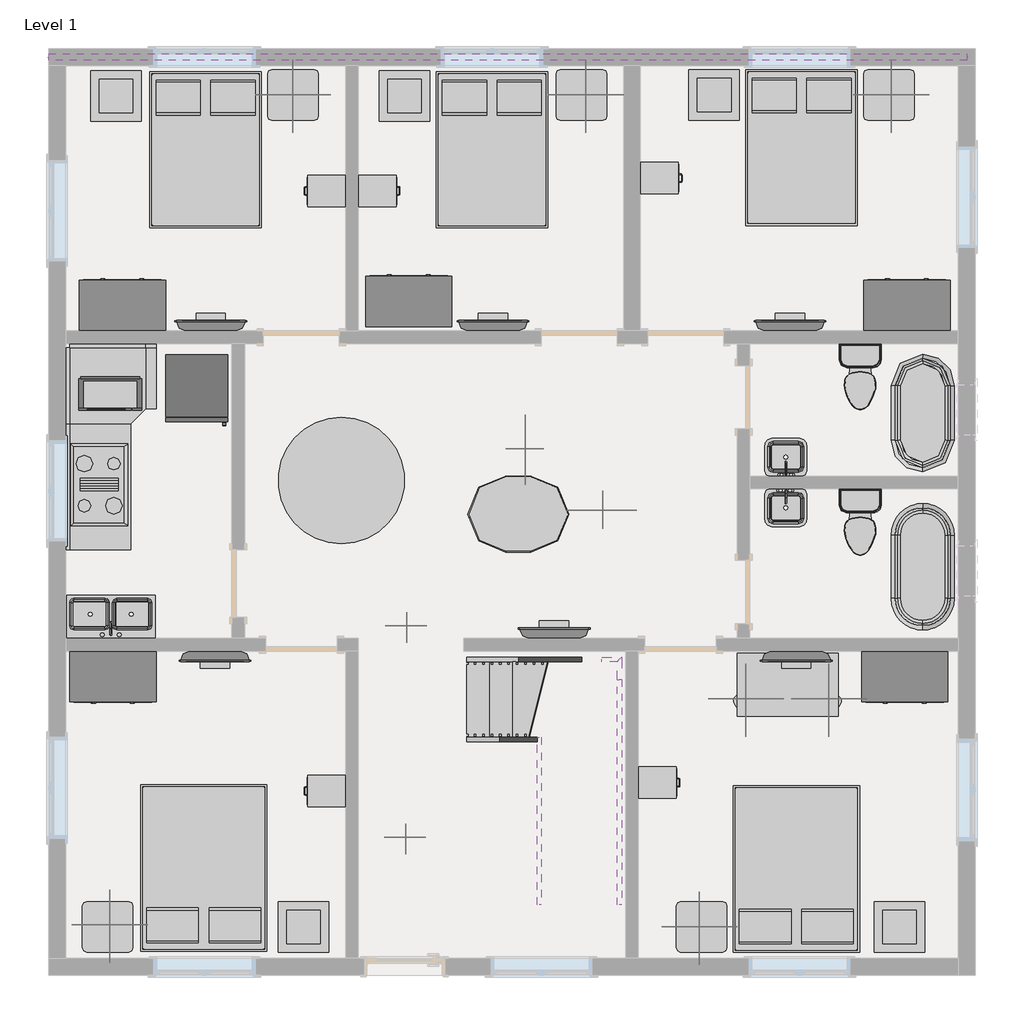
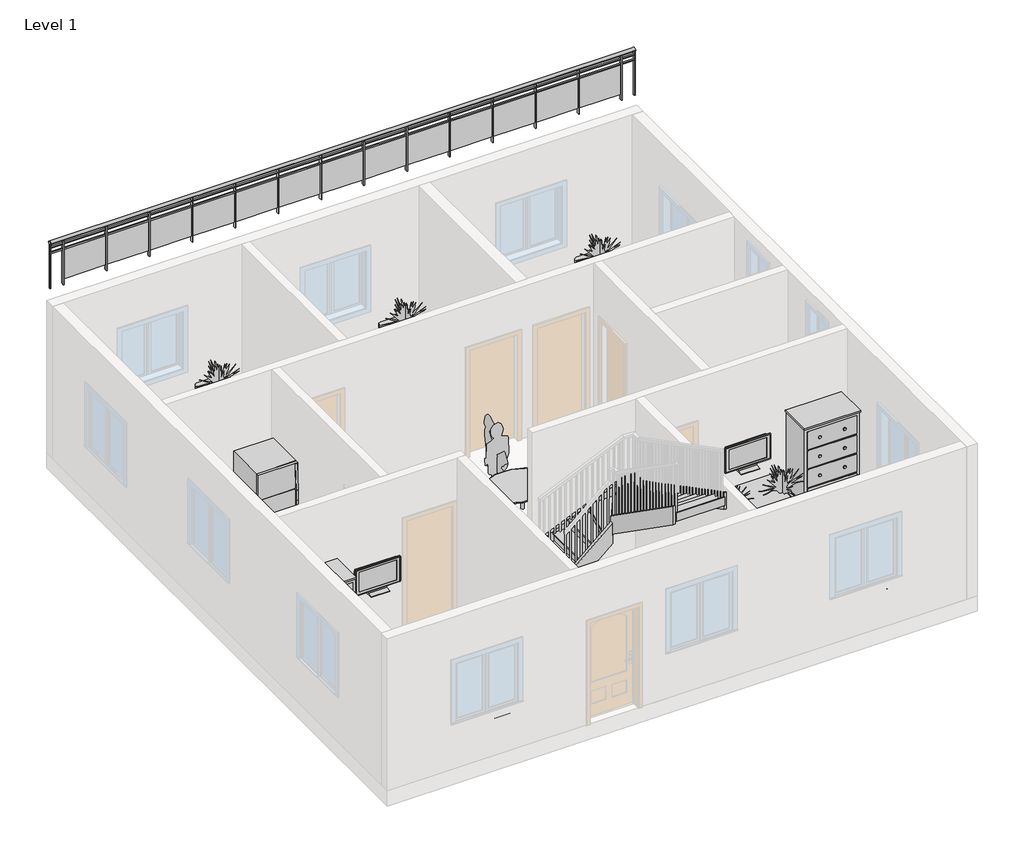
# One storey, part 3 of 3: 35 furniture elements, 9 flow terminals, 7 geographic elements, 7 proxies, 6 members, 1 railing, 1 stair flight.
"""IFC4 building model written with IfcOpenShell, lengths in millimetres."""

from ifc_helpers import new_model, si_unit, point, frame, origin, place, context, project, spatial, polyline, ellipse_curve, trimmed, outline, extrude, transform, mapped, element, save
from ifc_brep_helpers import plane_surface, extruded_surface, advanced_brep
from components import proxy_bb1e6e30, proxy_8a8d5ab2, rpc_female_69e001fa, rpc_male_28878092, proxy_a13a33b2, flow_terminal_2b63360b, flow_terminal_a53be723, flow_terminal_62a433f7, toilet_domestic_3d_toilet_domestic_3d_f7549cf7, toilet_domestic_3d_toilet_domestic_3d_183bbd19, flow_terminal_b374fae2, flow_terminal_a2f06f5b, furniture_c8abb964, furniture_1d2926bd, furniture_bb55ed6b, furniture_f72bdee3, furniture_56245f3a, furniture_b5c51a22, furniture_be1c6672, furniture_bbcc68ce, furniture_31d08a24, furniture_3f969c1c, furniture_6e13c3ce, rpc_plant_tropical_agave_1_5_93a2a214, stair_flight_d6903057

model = new_model("IFC4")

# Units and contexts
model_context = context("Model", 3, world=origin())
ifc_project = project(units=[si_unit("LENGTHUNIT", "METRE", prefix="MILLI")], contexts=[model_context])

# Site, building, storey
site = spatial("IfcSite", under=ifc_project)
building = spatial("IfcBuilding", under=site)
storey = spatial("IfcBuildingStorey", under=building, Name="Level 1", Elevation=0.0)

# Proxies
placement = place(None, origin())
proxy_shape = proxy_bb1e6e30(model_context)
element("IfcBuildingElementProxy", 1, Name="Cook Top-4 Unit : 36\" x 20\"", ObjectType="Cook Top-4 Unit : 36\" x 20\"", at=placement, inside=storey, context=model_context, shape_type="MappedRepresentation", body=[
    mapped(proxy_shape, transform((-16950.3067057, 8152.5187882, 0.0), x_axis=(0.0, 1.0000000000000002, 0.0), y_axis=(-1.0000000000000002, 0.0, 0.0), z_axis=(0.0, 0.0, 1.0))),
])
proxy_2_shape = proxy_8a8d5ab2(model_context)
element("IfcBuildingElementProxy", 2, Name="Microwave : 30\" x 16\" x 18\"", ObjectType="Microwave : 30\" x 16\" x 18\"", at=placement, inside=storey, context=model_context, shape_type="MappedRepresentation", body=[
    mapped(proxy_2_shape, transform((-17317.249583, 9604.149294, 0.0), x_axis=(1.0000000000000004, 0.0, 0.0), y_axis=(0.0, 1.0000000000000004, 0.0), z_axis=(0.0, 0.0, 1.0))),
])
rpc_female_shape = rpc_female_69e001fa(model_context)
element("IfcBuildingElementProxy", 3, Name="RPC Female", ObjectType="RPC Female", at=placement, inside=storey, context=model_context, shape_type="MappedRepresentation", body=[
    mapped(rpc_female_shape, transform((-11819.5067057, 8425.5687882, 0.0), x_axis=(1.0, 0.0, 0.0), y_axis=(0.0, 1.0, 0.0), z_axis=(0.0, 0.0, 1.0))),
])
element("IfcBuildingElementProxy", 4, Name="RPC Female", ObjectType="RPC Female", at=placement, inside=storey, context=model_context, shape_type="MappedRepresentation", body=[
    mapped(rpc_female_shape, transform((-11038.4567057, 7850.8434832, 0.0), x_axis=(0.0, -1.0000000000000004, 0.0), y_axis=(1.0000000000000004, 0.0, 0.0), z_axis=(0.0, 0.0, 1.0))),
])
rpc_male_shape = rpc_male_28878092(model_context)
element("IfcBuildingElementProxy", 5, Name="RPC Male", ObjectType="RPC Male", at=placement, inside=storey, context=model_context, shape_type="MappedRepresentation", body=[
    mapped(rpc_male_shape, transform((-13267.3067057, 3901.1937882, 0.0), x_axis=(1.0000000000000009, 0.0, 0.0), y_axis=(0.0, 1.0000000000000009, 0.0), z_axis=(0.0, 0.0, 1.0))),
])
element("IfcBuildingElementProxy", 6, Name="RPC Male", ObjectType="RPC Male", at=placement, inside=storey, context=model_context, shape_type="MappedRepresentation", body=[
    mapped(rpc_male_shape, transform((-13253.1160896, 6450.7187882, 0.0), x_axis=(1.0000000000000009, 0.0, 0.0), y_axis=(0.0, 1.0000000000000009, 0.0), z_axis=(0.0, 0.0, 1.0))),
])
proxy_3_shape = proxy_a13a33b2(model_context)
element("IfcBuildingElementProxy", 7, Name="Refrigerator : 30\" x 32\" RH", ObjectType="Refrigerator : 30\" x 32\" RH", at=placement, inside=storey, context=model_context, shape_type="MappedRepresentation", body=[
    mapped(proxy_3_shape, transform((-15774.3577342, 9328.8562882, 0.0), x_axis=(1.0000000000000007, 0.0, 0.0), y_axis=(0.0, 1.0000000000000007, 0.0), z_axis=(0.0, 0.0, 1.0))),
])

# Flow terminals
flow_terminal_shape = flow_terminal_2b63360b(model_context)
element("IfcFlowTerminal", 8, ObjectType="Floor Drain - Rectangular : 5\"x5\" Strainer - 2\" Drain", at=placement, inside=storey, context=model_context, shape_type="MappedRepresentation", body=[
    mapped(flow_terminal_shape, transform((-7692.0067057, 6552.3187882, 0.0), x_axis=(1.0, 0.0, 0.0), y_axis=(0.0, 1.0, 0.0), z_axis=(0.0, 0.0, 1.0))),
])
element("IfcFlowTerminal", 9, ObjectType="Floor Drain - Rectangular : 5\"x5\" Strainer - 2\" Drain", at=placement, inside=storey, context=model_context, shape_type="MappedRepresentation", body=[
    mapped(flow_terminal_shape, transform((-7628.5067057, 8457.3187882, 0.0), x_axis=(1.0, 0.0, 0.0), y_axis=(0.0, 1.0, 0.0), z_axis=(0.0, 0.0, 1.0))),
])
flow_terminal_2_shape = flow_terminal_a53be723(model_context)
element("IfcFlowTerminal", 10, ObjectType="Sink Kitchen-Double : 42\" x 21\"", at=placement, inside=storey, context=model_context, shape_type="MappedRepresentation", body=[
    mapped(flow_terminal_2_shape, transform((-16794.9174651, 6554.6641893, 0.0), x_axis=(-1.0000000000000002, 0.0, 0.0), y_axis=(0.0, -1.0000000000000002, 0.0), z_axis=(0.0, 0.0, 1.0))),
])
flow_terminal_3_shape = flow_terminal_62a433f7(model_context)
element("IfcFlowTerminal", 11, ObjectType="Sink Vanity-Square : 20\" x 18\"", at=placement, inside=storey, context=model_context, shape_type="MappedRepresentation", body=[
    mapped(flow_terminal_3_shape, transform((-8685.5959463, 7921.5733871, 0.0), x_axis=(1.0, 0.0, 0.0), y_axis=(0.0, 1.0, 0.0), z_axis=(0.0, 0.0, 1.0))),
])
element("IfcFlowTerminal", 12, ObjectType="Sink Vanity-Square : 20\" x 18\"", at=placement, inside=storey, context=model_context, shape_type="MappedRepresentation", body=[
    mapped(flow_terminal_3_shape, transform((-8654.2174651, 8434.2641893, 0.0), x_axis=(-1.0000000000000002, 0.0, 0.0), y_axis=(0.0, -1.0000000000000002, 0.0), z_axis=(0.0, 0.0, 1.0))),
])
toilet_domestic_3d_toilet_domestic_3d_shape = toilet_domestic_3d_toilet_domestic_3d_f7549cf7(model_context)
toilet_domestic_3d_toilet_domestic_3d_2_shape = toilet_domestic_3d_toilet_domestic_3d_183bbd19(model_context)
element("IfcFlowTerminal", 13, ObjectType="Toilet-Domestic-3D : Toilet-Domestic-3D", at=placement, inside=storey, context=model_context, shape_type="MappedRepresentation", body=[
    mapped(toilet_domestic_3d_toilet_domestic_3d_shape, transform((-7773.2107741, 7607.0227608, 0.0), x_axis=(1.0, 0.0, 0.0), y_axis=(0.0, 1.0, 0.0), z_axis=(0.0, 0.0, 1.0))),
    mapped(toilet_domestic_3d_toilet_domestic_3d_2_shape, transform((-7773.2107741, 7607.0227608, 0.0), x_axis=(1.0, 0.0, 0.0), y_axis=(0.0, 1.0, 0.0), z_axis=(0.0, 0.0, 1.0))),
])
element("IfcFlowTerminal", 14, ObjectType="Toilet-Domestic-3D : Toilet-Domestic-3D", at=placement, inside=storey, context=model_context, shape_type="MappedRepresentation", body=[
    mapped(toilet_domestic_3d_toilet_domestic_3d_shape, transform((-7773.2107741, 9359.6227608, 0.0), x_axis=(1.0, 0.0, 0.0), y_axis=(0.0, 1.0, 0.0), z_axis=(0.0, 0.0, 1.0))),
    mapped(toilet_domestic_3d_toilet_domestic_3d_2_shape, transform((-7773.2107741, 9359.6227608, 0.0), x_axis=(1.0, 0.0, 0.0), y_axis=(0.0, 1.0, 0.0), z_axis=(0.0, 0.0, 1.0))),
])
flow_terminal_4_shape = flow_terminal_b374fae2(model_context)
element("IfcFlowTerminal", 15, ObjectType="Tub-Free Standing-3D : 30\" x 60\"", at=placement, inside=storey, context=model_context, shape_type="MappedRepresentation", body=[
    mapped(flow_terminal_4_shape, transform((-7018.9067057, 7161.9187882, 0.0), x_axis=(1.0, 0.0, 0.0), y_axis=(0.0, 1.0, 0.0), z_axis=(0.0, 0.0, 1.0))),
])
flow_terminal_5_shape = flow_terminal_a2f06f5b(model_context)
element("IfcFlowTerminal", 16, ObjectType="Tub-Free Standing-3D : 30\" x 60\" 2", at=placement, inside=storey, context=model_context, shape_type="MappedRepresentation", body=[
    mapped(flow_terminal_5_shape, transform((-7018.9067057, 9016.1187882, 0.0), x_axis=(1.0, 0.0, 0.0), y_axis=(0.0, 1.0, 0.0), z_axis=(0.0, 0.0, 1.0))),
])

# Furniture
furniture_shape = furniture_c8abb964(model_context)
element("IfcFurniture", 17, ObjectType="Bed-Box : Double 53\" x 74\"", at=placement, inside=storey, context=model_context, shape_type="MappedRepresentation", body=[
    mapped(furniture_shape, transform((-16006.7591647, 12425.5482964, 0.0), x_axis=(1.0, 0.0, 0.0), y_axis=(0.0, 1.0, 0.0), z_axis=(0.0, 0.0, 1.0))),
])
element("IfcFurniture", 18, ObjectType="Bed-Box : Double 53\" x 74\"", at=placement, inside=storey, context=model_context, shape_type="MappedRepresentation", body=[
    mapped(furniture_shape, transform((-12552.3591647, 12425.5482964, 0.0), x_axis=(1.0, 0.0, 0.0), y_axis=(0.0, 1.0, 0.0), z_axis=(0.0, 0.0, 1.0))),
])
element("IfcFurniture", 19, ObjectType="Bed-Box : Double 53\" x 74\"", at=placement, inside=storey, context=model_context, shape_type="MappedRepresentation", body=[
    mapped(furniture_shape, transform((-8818.5591647, 12450.9482964, 0.0), x_axis=(1.0, 0.0, 0.0), y_axis=(0.0, 1.0, 0.0), z_axis=(0.0, 0.0, 1.0))),
])
furniture_2_shape = furniture_1d2926bd(model_context)
element("IfcFurniture", 20, ObjectType="Bed-Box : Queen 60\" x 79\"", at=placement, inside=storey, context=model_context, shape_type="MappedRepresentation", body=[
    mapped(furniture_2_shape, transform((-15350.1067057, 3295.28928, 0.0), x_axis=(-1.0000000000000002, 0.0, 0.0), y_axis=(0.0, -1.0000000000000002, 0.0), z_axis=(0.0, 0.0, 1.0))),
])
element("IfcFurniture", 21, ObjectType="Bed-Box : Queen 60\" x 79\"", at=placement, inside=storey, context=model_context, shape_type="MappedRepresentation", body=[
    mapped(furniture_2_shape, transform((-8203.7542467, 3282.58928, 0.0), x_axis=(-1.0, 0.0, 0.0), y_axis=(0.0, -1.0, 0.0), z_axis=(0.0, 0.0, 1.0))),
])
furniture_3_shape = furniture_bb55ed6b(model_context)
element("IfcFurniture", 22, ObjectType="Cabinet-File 2 Drawer : 15\" x 18\"", at=placement, inside=storey, context=model_context, shape_type="MappedRepresentation", body=[
    mapped(furniture_3_shape, transform((-14064.9724056, 11564.7774513, 0.0), x_axis=(0.0, -1.0000000000000002, 0.0), y_axis=(1.0000000000000002, 0.0, 0.0), z_axis=(0.0, 0.0, 1.0))),
])
element("IfcFurniture", 23, ObjectType="Cabinet-File 2 Drawer : 15\" x 18\"", at=placement, inside=storey, context=model_context, shape_type="MappedRepresentation", body=[
    mapped(furniture_3_shape, transform((-13739.6410058, 11823.7152352, 0.0), x_axis=(0.0, 1.0, 0.0), y_axis=(-1.0, 0.0, 0.0), z_axis=(0.0, 0.0, 1.0))),
])
element("IfcFurniture", 24, ObjectType="Cabinet-File 2 Drawer : 15\" x 18\"", at=placement, inside=storey, context=model_context, shape_type="MappedRepresentation", body=[
    mapped(furniture_3_shape, transform((-10336.0410058, 11976.1152352, 0.0), x_axis=(0.0, 1.0000000000000002, 0.0), y_axis=(-1.0000000000000002, 0.0, 0.0), z_axis=(0.0, 0.0, 1.0))),
])
element("IfcFurniture", 25, ObjectType="Cabinet-File 2 Drawer : 15\" x 18\"", at=placement, inside=storey, context=model_context, shape_type="MappedRepresentation", body=[
    mapped(furniture_3_shape, transform((-14064.9724056, 4328.9223411, 0.0), x_axis=(0.0, -1.0000000000000007, 0.0), y_axis=(1.0000000000000007, 0.0, 0.0), z_axis=(0.0, 0.0, 1.0))),
])
element("IfcFurniture", 26, ObjectType="Cabinet-File 2 Drawer : 15\" x 18\"", at=placement, inside=storey, context=model_context, shape_type="MappedRepresentation", body=[
    mapped(furniture_3_shape, transform((-10361.4410058, 4686.3152352, 0.0), x_axis=(0.0, 1.0, 0.0), y_axis=(-1.0, 0.0, 0.0), z_axis=(0.0, 0.0, 1.0))),
])
furniture_4_shape = furniture_f72bdee3(model_context)
element("IfcFurniture", 27, ObjectType="Dresser : 48\" x 72\" x 24\"", at=placement, inside=storey, context=model_context, shape_type="MappedRepresentation", body=[
    mapped(furniture_4_shape, transform((-16940.0999656, 9948.3558341, 0.0), x_axis=(-1.0000000000000004, 0.0, 0.0), y_axis=(0.0, -1.0000000000000004, 0.0), z_axis=(0.0, 0.0, 1.0))),
])
element("IfcFurniture", 28, ObjectType="Dresser : 48\" x 72\" x 24\"", at=placement, inside=storey, context=model_context, shape_type="MappedRepresentation", body=[
    mapped(furniture_4_shape, transform((-13485.6999656, 9999.1558341, 0.0), x_axis=(-1.0000000000000004, 0.0, 0.0), y_axis=(0.0, -1.0000000000000004, 0.0), z_axis=(0.0, 0.0, 1.0))),
])
element("IfcFurniture", 29, ObjectType="Dresser : 48\" x 72\" x 24\"", at=placement, inside=storey, context=model_context, shape_type="MappedRepresentation", body=[
    mapped(furniture_4_shape, transform((-7478.5999656, 9948.3558341, 0.0), x_axis=(-1.0000000000000004, 0.0, 0.0), y_axis=(0.0, -1.0000000000000004, 0.0), z_axis=(0.0, 0.0, 1.0))),
])
element("IfcFurniture", 30, ObjectType="Dresser : 48\" x 72\" x 24\"", at=placement, inside=storey, context=model_context, shape_type="MappedRepresentation", body=[
    mapped(furniture_4_shape, transform((-16516.0134459, 6204.2817423, 0.0), x_axis=(1.0, 0.0, 0.0), y_axis=(0.0, 1.0, 0.0), z_axis=(0.0, 0.0, 1.0))),
])
element("IfcFurniture", 31, ObjectType="Dresser : 48\" x 72\" x 24\"", at=placement, inside=storey, context=model_context, shape_type="MappedRepresentation", body=[
    mapped(furniture_4_shape, transform((-6965.6134459, 6204.2817423, 0.0), x_axis=(1.0, 0.0, 0.0), y_axis=(0.0, 1.0, 0.0), z_axis=(0.0, 0.0, 1.0))),
])
furniture_5_shape = furniture_56245f3a(model_context)
element("IfcFurniture", 32, ObjectType="TV - Flat Screen : 32\"", at=placement, inside=storey, context=model_context, shape_type="MappedRepresentation", body=[
    mapped(furniture_5_shape, transform((-15608.0512199, 10065.2574118, 990.6), x_axis=(-1.0000000000000002, 0.0, 0.0), y_axis=(0.0, -1.0000000000000002, 0.0), z_axis=(0.0, 0.0, 1.0))),
])
element("IfcFurniture", 33, ObjectType="TV - Flat Screen : 32\"", at=placement, inside=storey, context=model_context, shape_type="MappedRepresentation", body=[
    mapped(furniture_5_shape, transform((-12204.4512199, 10065.2574118, 990.6), x_axis=(-1.0000000000000009, 0.0, 0.0), y_axis=(0.0, -1.0000000000000009, 0.0), z_axis=(0.0, 0.0, 1.0))),
])
element("IfcFurniture", 34, ObjectType="TV - Flat Screen : 32\"", at=placement, inside=storey, context=model_context, shape_type="MappedRepresentation", body=[
    mapped(furniture_5_shape, transform((-8623.0512199, 10065.2574118, 990.6), x_axis=(-1.0, 0.0, 0.0), y_axis=(0.0, -1.0, 0.0), z_axis=(0.0, 0.0, 1.0))),
])
element("IfcFurniture", 35, ObjectType="TV - Flat Screen : 32\"", at=placement, inside=storey, context=model_context, shape_type="MappedRepresentation", body=[
    mapped(furniture_5_shape, transform((-15549.3621916, 6087.3801645, 990.6), x_axis=(1.0, 0.0, 0.0), y_axis=(0.0, 1.0, 0.0), z_axis=(0.0, 0.0, 1.0))),
])
element("IfcFurniture", 36, ObjectType="TV - Flat Screen : 32\"", at=placement, inside=storey, context=model_context, shape_type="MappedRepresentation", body=[
    mapped(furniture_5_shape, transform((-8538.9621916, 6087.3801645, 990.6), x_axis=(1.0, 0.0, 0.0), y_axis=(0.0, 1.0, 0.0), z_axis=(0.0, 0.0, 1.0))),
])
element("IfcFurniture", 37, ObjectType="TV - Flat Screen : 32\"", at=placement, inside=storey, context=model_context, shape_type="MappedRepresentation", body=[
    mapped(furniture_5_shape, transform((-11467.8512199, 6356.8574118, 1092.2), x_axis=(-1.0000000000000002, 0.0, 0.0), y_axis=(0.0, -1.0000000000000002, 0.0), z_axis=(0.0, 0.0, 1.0))),
])
furniture_6_shape = furniture_b5c51a22(model_context)
element("IfcFurniture", 38, ObjectType="Table-Coffee : 24\" x 24\" x 24\"", at=placement, inside=storey, context=model_context, shape_type="MappedRepresentation", body=[
    mapped(furniture_6_shape, transform((-16765.3724724, 12743.6077104, 0.0), x_axis=(1.0, 0.0, 0.0), y_axis=(0.0, 1.0, 0.0), z_axis=(0.0, 0.0, 1.0))),
])
element("IfcFurniture", 39, ObjectType="Table-Coffee : 24\" x 24\" x 24\"", at=placement, inside=storey, context=model_context, shape_type="MappedRepresentation", body=[
    mapped(furniture_6_shape, transform((-13285.5724724, 12743.6077104, 0.0), x_axis=(1.0, 0.0, 0.0), y_axis=(0.0, 1.0, 0.0), z_axis=(0.0, 0.0, 1.0))),
])
element("IfcFurniture", 40, ObjectType="Table-Coffee : 24\" x 24\" x 24\"", at=placement, inside=storey, context=model_context, shape_type="MappedRepresentation", body=[
    mapped(furniture_6_shape, transform((-9551.7724724, 12756.3077104, 0.0), x_axis=(1.0, 0.0, 0.0), y_axis=(0.0, 1.0, 0.0), z_axis=(0.0, 0.0, 1.0))),
])
element("IfcFurniture", 41, ObjectType="Table-Coffee : 24\" x 24\" x 24\"", at=placement, inside=storey, context=model_context, shape_type="MappedRepresentation", body=[
    mapped(furniture_6_shape, transform((-14504.7724724, 2723.3077104, 0.0), x_axis=(1.0, 0.0, 0.0), y_axis=(0.0, 1.0, 0.0), z_axis=(0.0, 0.0, 1.0))),
])
element("IfcFurniture", 42, ObjectType="Table-Coffee : 24\" x 24\" x 24\"", at=placement, inside=storey, context=model_context, shape_type="MappedRepresentation", body=[
    mapped(furniture_6_shape, transform((-7316.5724724, 2723.3077104, 0.0), x_axis=(1.0, 0.0, 0.0), y_axis=(0.0, 1.0, 0.0), z_axis=(0.0, 0.0, 1.0))),
])
furniture_7_shape = furniture_be1c6672(model_context)
element("IfcFurniture", 43, ObjectType="Table-Dining Oval : 36\" x 48\"", at=placement, inside=storey, context=model_context, shape_type="MappedRepresentation", body=[
    mapped(furniture_7_shape, transform((-11493.8870336, 8155.0171488, 0.0), x_axis=(1.0, 0.0, 0.0), y_axis=(0.0, 1.0, 0.0), z_axis=(0.0, 0.0, 1.0))),
])
furniture_8_shape = furniture_bbcc68ce(model_context)
element("IfcFurniture", 44, ObjectType="Table-Dining Round w Chairs : 60\" Diameter", at=placement, inside=storey, context=model_context, shape_type="MappedRepresentation", body=[
    mapped(furniture_8_shape, transform((-14132.9886729, 8388.1974767, 0.0), x_axis=(1.0, 0.0, 0.0), y_axis=(0.0, 1.0, 0.0), z_axis=(0.0, 0.0, 1.0))),
])
furniture_9_shape = furniture_31d08a24(model_context)
element("IfcFurniture", 45, ObjectType="Table-End : 24\" x 24\"", at=placement, inside=storey, context=model_context, shape_type="MappedRepresentation", body=[
    mapped(furniture_9_shape, transform((-14922.040336, 12699.1187882, 0.0), x_axis=(1.0, 0.0, 0.0), y_axis=(0.0, 1.0, 0.0), z_axis=(0.0, 0.0, 1.0))),
])
element("IfcFurniture", 46, ObjectType="Table-End : 24\" x 24\"", at=placement, inside=storey, context=model_context, shape_type="MappedRepresentation", body=[
    mapped(furniture_9_shape, transform((-11442.240336, 12699.1187882, 0.0), x_axis=(1.0, 0.0, 0.0), y_axis=(0.0, 1.0, 0.0), z_axis=(0.0, 0.0, 1.0))),
])
element("IfcFurniture", 47, ObjectType="Table-End : 24\" x 24\"", at=placement, inside=storey, context=model_context, shape_type="MappedRepresentation", body=[
    mapped(furniture_9_shape, transform((-7733.840336, 12699.1187882, 0.0), x_axis=(1.0, 0.0, 0.0), y_axis=(0.0, 1.0, 0.0), z_axis=(0.0, 0.0, 1.0))),
])
element("IfcFurniture", 48, ObjectType="Table-End : 24\" x 24\"", at=placement, inside=storey, context=model_context, shape_type="MappedRepresentation", body=[
    mapped(furniture_9_shape, transform((-17157.240336, 2666.1187882, 0.0), x_axis=(1.0, 0.0, 0.0), y_axis=(0.0, 1.0, 0.0), z_axis=(0.0, 0.0, 1.0))),
])
element("IfcFurniture", 49, ObjectType="Table-End : 24\" x 24\"", at=placement, inside=storey, context=model_context, shape_type="MappedRepresentation", body=[
    mapped(furniture_9_shape, transform((-9994.440336, 2666.1187882, 0.0), x_axis=(1.0, 0.0, 0.0), y_axis=(0.0, 1.0, 0.0), z_axis=(0.0, 0.0, 1.0))),
])
furniture_10_shape = furniture_3f969c1c(model_context)
element("IfcFurniture", 50, ObjectType="Table-Rectangular : 72\" x 30\"", at=placement, inside=storey, context=model_context, shape_type="MappedRepresentation", body=[
    mapped(furniture_10_shape, transform((-8644.5067057, 5739.5187882, 0.0), x_axis=(1.0, 0.0, 0.0), y_axis=(0.0, 1.0, 0.0), z_axis=(0.0, 0.0, 1.0))),
])
furniture_11_shape = furniture_6e13c3ce(model_context)
element("IfcFurniture", 51, ObjectType="Work Station Cubicle : 96\" x 96\"", at=placement, inside=storey, context=model_context, shape_type="MappedRepresentation", body=[
    mapped(furniture_11_shape, transform((-17224.9749535, 10349.3417958, 0.0), x_axis=(1.0, 0.0, 0.0), y_axis=(0.0, 1.0, 0.0), z_axis=(0.0, 0.0, 1.0))),
])

# Geographic elements
rpc_plant_tropical_agave_1_5_shape = rpc_plant_tropical_agave_1_5_93a2a214(model_context)
element("IfcGeographicElement", 52, ObjectType="RPC Plant - Tropical : Agave - 1.5'", at=placement, inside=storey, context=model_context, shape_type="MappedRepresentation", body=[
    mapped(rpc_plant_tropical_agave_1_5_shape, transform((-14613.5067057, 12851.5187882, 609.6), x_axis=(1.0, 0.0, 0.0), y_axis=(0.0, 1.0, 0.0), z_axis=(0.0, 0.0, 1.0))),
])
element("IfcGeographicElement", 53, ObjectType="RPC Plant - Tropical : Agave - 1.5'", at=placement, inside=storey, context=model_context, shape_type="MappedRepresentation", body=[
    mapped(rpc_plant_tropical_agave_1_5_shape, transform((-11082.9067057, 12851.5187882, 609.6), x_axis=(1.0, 0.0, 0.0), y_axis=(0.0, 1.0, 0.0), z_axis=(0.0, 0.0, 1.0))),
])
element("IfcGeographicElement", 54, ObjectType="RPC Plant - Tropical : Agave - 1.5'", at=placement, inside=storey, context=model_context, shape_type="MappedRepresentation", body=[
    mapped(rpc_plant_tropical_agave_1_5_shape, transform((-7399.9067057, 12851.5187882, 609.6), x_axis=(1.0, 0.0, 0.0), y_axis=(0.0, 1.0, 0.0), z_axis=(0.0, 0.0, 1.0))),
])
element("IfcGeographicElement", 55, ObjectType="RPC Plant - Tropical : Agave - 1.5'", at=placement, inside=storey, context=model_context, shape_type="MappedRepresentation", body=[
    mapped(rpc_plant_tropical_agave_1_5_shape, transform((-16823.3067057, 2843.9187882, 609.6), x_axis=(1.0, 0.0, 0.0), y_axis=(0.0, 1.0, 0.0), z_axis=(0.0, 0.0, 1.0))),
])
element("IfcGeographicElement", 56, ObjectType="RPC Plant - Tropical : Agave - 1.5'", at=placement, inside=storey, context=model_context, shape_type="MappedRepresentation", body=[
    mapped(rpc_plant_tropical_agave_1_5_shape, transform((-9711.3067057, 2818.5187882, 609.6), x_axis=(1.0, 0.0, 0.0), y_axis=(0.0, 1.0, 0.0), z_axis=(0.0, 0.0, 1.0))),
])
element("IfcGeographicElement", 57, ObjectType="RPC Plant - Tropical : Agave - 1.5'", at=placement, inside=storey, context=model_context, shape_type="MappedRepresentation", body=[
    mapped(rpc_plant_tropical_agave_1_5_shape, transform((-8149.2067057, 5568.0687882, 660.4), x_axis=(1.0, 0.0, 0.0), y_axis=(0.0, 1.0, 0.0), z_axis=(0.0, 0.0, 1.0))),
])
element("IfcGeographicElement", 58, ObjectType="RPC Plant - Tropical : Agave - 1.5'", at=placement, inside=storey, context=model_context, shape_type="MappedRepresentation", body=[
    mapped(rpc_plant_tropical_agave_1_5_shape, transform((-9152.5067057, 5568.0687882, 660.4), x_axis=(1.0, 0.0, 0.0), y_axis=(0.0, 1.0, 0.0), z_axis=(0.0, 0.0, 1.0))),
])

# Members
element("IfcMember", 59, ObjectType="Stringer - 2\" Width", at=placement, inside=storey, context=model_context, shape_type="SweptSolid", body=[
    extrude(outline(polyline([(922.8849999, -12520.2436952), (590.0562463, -12520.2436952), (1305.2683876, -10889.5815024), (1638.0971411, -10889.5815024), (922.8849999, -12520.2436952)])), frame((0.0, 6018.9187882, 0.0), z_axis=(0.0, 1.0, 0.0), x_axis=(0.0, 0.0, 1.0)), (0.0, 0.0, 1.0), 50.8),
])
element("IfcMember", 60, ObjectType="Stringer - 2\" Width", at=placement, inside=storey, context=model_context, shape_type="SweptSolid", body=[
    extrude(outline(polyline([(-10889.5815024, 6018.9187882), (-10889.5815024, 6069.7187882), (-10651.1067057, 6069.7187882), (-10701.9067057, 6018.9187882), (-10889.5815024, 6018.9187882)])), frame((0.0, 0.0, 1305.2683876), z_axis=(0.0, 0.0, 1.0), x_axis=(1.0, 0.0, 0.0)), (0.0, 0.0, 1.0), 332.8287535),
])
element("IfcMember", 61, ObjectType="Stringer - 2\" Width", at=placement, inside=storey, context=model_context, shape_type="SweptSolid", body=[
    extrude(outline(polyline([(-10701.9067057, 6018.9187882), (-10651.1067057, 6069.7187882), (-10651.1067057, 5800.7654451), (-10701.9067057, 5800.7654451), (-10701.9067057, 6018.9187882)])), frame((0.0, 0.0, 1305.2683876), z_axis=(0.0, 0.0, 1.0), x_axis=(1.0, 0.0, 0.0)), (0.0, 0.0, 1.0), 332.8287535),
])
element("IfcMember", 62, ObjectType="Stringer - 2\" Width", at=placement, inside=storey, context=model_context, shape_type="SweptSolid", body=[
    extrude(outline(polyline([(5800.7654451, 1638.0971411), (5800.7654451, 1305.2683876), (3082.9817987, 2720.7901969), (3082.9817987, 3053.6189504), (5800.7654451, 1638.0971411)])), frame((-10701.9067057, 0.0, 0.0), z_axis=(1.0, 0.0, 0.0), x_axis=(0.0, 1.0, 0.0)), (0.0, 0.0, 1.0), 50.8),
])
element("IfcMember", 63, ObjectType="Stringer - 2\" Width", at=placement, inside=storey, context=model_context, shape_type="SweptSolid", body=[
    extrude(outline(polyline([(842.634734, -12520.2436952), (435.4922729, -12520.2436952), (1191.0265733, -11667.1067057), (1598.1690344, -11667.1067057), (842.634734, -12520.2436952)])), frame((0.0, 5053.7187882, 0.0), z_axis=(0.0, 1.0, 0.0), x_axis=(0.0, 0.0, 1.0)), (0.0, 0.0, 1.0), 50.8),
])
element("IfcMember", 64, ObjectType="Stringer - 2\" Width", at=placement, inside=storey, context=model_context, shape_type="SweptSolid", body=[
    extrude(outline(polyline([(5104.5187882, 1709.9296678), (5104.5187882, 1337.7212805), (3082.9817987, 2754.5609981), (3082.9817987, 3126.7693854), (5104.5187882, 1709.9296678)])), frame((-11667.1067057, 0.0, 0.0), z_axis=(1.0, 0.0, 0.0), x_axis=(0.0, 1.0, 0.0)), (0.0, 0.0, 1.0), 50.8),
])

# Railing
element("IfcRailing", 65, ObjectType="Glass Panel - Bottom Fill", at=placement, inside=storey, context=model_context, shape_type="SolidModel", body=[
    advanced_brep(
    [(-17559.9067057, 13346.8187882, 4267.2), (-17559.9067057, 13270.6187882, 4267.2), (-6485.5067057, 13346.8187882, 4267.2), (-6485.5067057, 13270.6187882, 4267.2)],
    [
        (0, 1, ellipse_curve(frame((-17559.9067057, 13308.7187882, 4267.2), z_axis=(-1.0, 0.0, 0.0), x_axis=(0.0, -1.0, 0.0)), 38.1, 28.575)),
        (1, 0, ellipse_curve(frame((-17559.9067057, 13308.7187882, 4267.2), z_axis=(-1.0, 0.0, 0.0), x_axis=(0.0, -1.0, 0.0)), 38.1, 28.575)),
        (2, 3, ellipse_curve(frame((-6485.5067057, 13308.7187882, 4267.2), z_axis=(1.0, 0.0, 0.0), x_axis=(0.0, -1.0, 0.0)), 38.1, 28.575)),
        (3, 2, ellipse_curve(frame((-6485.5067057, 13308.7187882, 4267.2), z_axis=(1.0, 0.0, 0.0), x_axis=(0.0, -1.0, 0.0)), 38.1, 28.575)),
        (0, 2),
        (3, 1),
    ],
    [
        plane_surface(frame((-17559.9067057, 13308.7187882, 4267.2), z_axis=(-1.0, 0.0, 0.0), x_axis=(0.0, 1.0, 0.0))),
        plane_surface(frame((-6485.5067057, 13308.7187882, 4267.2), z_axis=(1.0, 0.0, 0.0), x_axis=(0.0, 1.0, 0.0))),
        extruded_surface(trimmed(ellipse_curve(frame((-6485.5067057, 13308.7187882, 4267.2), z_axis=(-1.0, 0.0, 0.0), x_axis=(0.0, -1.0, 0.0)), 38.1, 28.575), [point((-6485.5067057, 13346.8187882, 4267.2))], [point((-6485.5067057, 13270.6187882, 4267.2))], True, "CARTESIAN"), (-11074.4, 0.0, 0.0), 11074.4),
        extruded_surface(trimmed(ellipse_curve(frame((-6485.5067057, 13308.7187882, 4267.2), z_axis=(-1.0, 0.0, 0.0), x_axis=(0.0, -1.0, 0.0)), 38.1, 28.575), [point((-6485.5067057, 13270.6187882, 4267.2))], [point((-6485.5067057, 13346.8187882, 4267.2))], True, "CARTESIAN"), (-11074.4, 0.0, 0.0), 11074.4),
    ],
    [
        (0, [[1, 2]]),
        (1, [[3, 4]]),
        (2, [[-1, 5, -4, 6]]),
        (3, [[-2, -6, -3, -5]]),
    ],
),
    extrude(outline(polyline([(-17559.9067057, 13296.0187882), (-17559.9067057, 13321.4187882), (-6485.5067057, 13321.4187882), (-6485.5067057, 13296.0187882), (-17559.9067057, 13296.0187882)])), frame((0.0, 0.0, 4152.9), z_axis=(0.0, 0.0, 1.0), x_axis=(1.0, 0.0, 0.0)), (0.0, 0.0, 1.0), 25.4),
    extrude(outline(polyline([(-17559.9067057, 13296.0187882), (-17559.9067057, 13321.4187882), (-6485.5067057, 13321.4187882), (-6485.5067057, 13296.0187882), (-17559.9067057, 13296.0187882)])), frame((0.0, 0.0, 4051.3), z_axis=(0.0, 0.0, 1.0), x_axis=(1.0, 0.0, 0.0)), (0.0, 0.0, 1.0), 25.4),
    extrude(outline(polyline([(-6745.8567057, 13283.3187882), (-6745.8567057, 13334.1187882), (-6733.1567057, 13334.1187882), (-6733.1567057, 13283.3187882), (-6745.8567057, 13283.3187882)])), frame((0.0, 0.0, 3352.8), z_axis=(0.0, 0.0, 1.0), x_axis=(1.0, 0.0, 0.0)), (0.0, 0.0, 1.0), 885.6788223),
    extrude(outline(polyline([(-7552.3067057, 13315.2539452), (-6739.5067057, 13315.2539452), (-6739.5067057, 13308.9039452), (-7552.3067057, 13308.9039452), (-7552.3067057, 13315.2539452)])), frame((0.0, 0.0, 3454.4), z_axis=(0.0, 0.0, 1.0), x_axis=(1.0, 0.0, 0.0)), (0.0, 0.0, 1.0), 596.9),
    extrude(outline(polyline([(-7558.6567057, 13283.3187882), (-7558.6567057, 13334.1187882), (-7545.9567057, 13334.1187882), (-7545.9567057, 13283.3187882), (-7558.6567057, 13283.3187882)])), frame((0.0, 0.0, 3352.8), z_axis=(0.0, 0.0, 1.0), x_axis=(1.0, 0.0, 0.0)), (0.0, 0.0, 1.0), 885.6788223),
    extrude(outline(polyline([(-8365.1067057, 13315.2539452), (-7552.3067057, 13315.2539452), (-7552.3067057, 13308.9039452), (-8365.1067057, 13308.9039452), (-8365.1067057, 13315.2539452)])), frame((0.0, 0.0, 3454.4), z_axis=(0.0, 0.0, 1.0), x_axis=(1.0, 0.0, 0.0)), (0.0, 0.0, 1.0), 596.9),
    extrude(outline(polyline([(-8371.4567057, 13283.3187882), (-8371.4567057, 13334.1187882), (-8358.7567057, 13334.1187882), (-8358.7567057, 13283.3187882), (-8371.4567057, 13283.3187882)])), frame((0.0, 0.0, 3352.8), z_axis=(0.0, 0.0, 1.0), x_axis=(1.0, 0.0, 0.0)), (0.0, 0.0, 1.0), 885.6788223),
    extrude(outline(polyline([(-9177.9067057, 13315.2539452), (-8365.1067057, 13315.2539452), (-8365.1067057, 13308.9039452), (-9177.9067057, 13308.9039452), (-9177.9067057, 13315.2539452)])), frame((0.0, 0.0, 3454.4), z_axis=(0.0, 0.0, 1.0), x_axis=(1.0, 0.0, 0.0)), (0.0, 0.0, 1.0), 596.9),
    extrude(outline(polyline([(-9184.2567057, 13283.3187882), (-9184.2567057, 13334.1187882), (-9171.5567057, 13334.1187882), (-9171.5567057, 13283.3187882), (-9184.2567057, 13283.3187882)])), frame((0.0, 0.0, 3352.8), z_axis=(0.0, 0.0, 1.0), x_axis=(1.0, 0.0, 0.0)), (0.0, 0.0, 1.0), 885.6788223),
    extrude(outline(polyline([(-9990.7067057, 13315.2539452), (-9177.9067057, 13315.2539452), (-9177.9067057, 13308.9039452), (-9990.7067057, 13308.9039452), (-9990.7067057, 13315.2539452)])), frame((0.0, 0.0, 3454.4), z_axis=(0.0, 0.0, 1.0), x_axis=(1.0, 0.0, 0.0)), (0.0, 0.0, 1.0), 596.9),
    extrude(outline(polyline([(-9997.0567057, 13283.3187882), (-9997.0567057, 13334.1187882), (-9984.3567057, 13334.1187882), (-9984.3567057, 13283.3187882), (-9997.0567057, 13283.3187882)])), frame((0.0, 0.0, 3352.8), z_axis=(0.0, 0.0, 1.0), x_axis=(1.0, 0.0, 0.0)), (0.0, 0.0, 1.0), 885.6788223),
    extrude(outline(polyline([(-10803.5067057, 13315.2539452), (-9990.7067057, 13315.2539452), (-9990.7067057, 13308.9039452), (-10803.5067057, 13308.9039452), (-10803.5067057, 13315.2539452)])), frame((0.0, 0.0, 3454.4), z_axis=(0.0, 0.0, 1.0), x_axis=(1.0, 0.0, 0.0)), (0.0, 0.0, 1.0), 596.9),
    extrude(outline(polyline([(-10809.8567057, 13283.3187882), (-10809.8567057, 13334.1187882), (-10797.1567057, 13334.1187882), (-10797.1567057, 13283.3187882), (-10809.8567057, 13283.3187882)])), frame((0.0, 0.0, 3352.8), z_axis=(0.0, 0.0, 1.0), x_axis=(1.0, 0.0, 0.0)), (0.0, 0.0, 1.0), 885.6788223),
    extrude(outline(polyline([(-11616.3067057, 13315.2539452), (-10803.5067057, 13315.2539452), (-10803.5067057, 13308.9039452), (-11616.3067057, 13308.9039452), (-11616.3067057, 13315.2539452)])), frame((0.0, 0.0, 3454.4), z_axis=(0.0, 0.0, 1.0), x_axis=(1.0, 0.0, 0.0)), (0.0, 0.0, 1.0), 596.9),
    extrude(outline(polyline([(-11622.6567057, 13283.3187882), (-11622.6567057, 13334.1187882), (-11609.9567057, 13334.1187882), (-11609.9567057, 13283.3187882), (-11622.6567057, 13283.3187882)])), frame((0.0, 0.0, 3352.8), z_axis=(0.0, 0.0, 1.0), x_axis=(1.0, 0.0, 0.0)), (0.0, 0.0, 1.0), 885.6788223),
    extrude(outline(polyline([(-12429.1067057, 13315.2539452), (-11616.3067057, 13315.2539452), (-11616.3067057, 13308.9039452), (-12429.1067057, 13308.9039452), (-12429.1067057, 13315.2539452)])), frame((0.0, 0.0, 3454.4), z_axis=(0.0, 0.0, 1.0), x_axis=(1.0, 0.0, 0.0)), (0.0, 0.0, 1.0), 596.9),
    extrude(outline(polyline([(-12435.4567057, 13283.3187882), (-12435.4567057, 13334.1187882), (-12422.7567057, 13334.1187882), (-12422.7567057, 13283.3187882), (-12435.4567057, 13283.3187882)])), frame((0.0, 0.0, 3352.8), z_axis=(0.0, 0.0, 1.0), x_axis=(1.0, 0.0, 0.0)), (0.0, 0.0, 1.0), 885.6788223),
    extrude(outline(polyline([(-13241.9067057, 13315.2539452), (-12429.1067057, 13315.2539452), (-12429.1067057, 13308.9039452), (-13241.9067057, 13308.9039452), (-13241.9067057, 13315.2539452)])), frame((0.0, 0.0, 3454.4), z_axis=(0.0, 0.0, 1.0), x_axis=(1.0, 0.0, 0.0)), (0.0, 0.0, 1.0), 596.9),
    extrude(outline(polyline([(-13248.2567057, 13283.3187882), (-13248.2567057, 13334.1187882), (-13235.5567057, 13334.1187882), (-13235.5567057, 13283.3187882), (-13248.2567057, 13283.3187882)])), frame((0.0, 0.0, 3352.8), z_axis=(0.0, 0.0, 1.0), x_axis=(1.0, 0.0, 0.0)), (0.0, 0.0, 1.0), 885.6788223),
    extrude(outline(polyline([(-14054.7067057, 13315.2539452), (-13241.9067057, 13315.2539452), (-13241.9067057, 13308.9039452), (-14054.7067057, 13308.9039452), (-14054.7067057, 13315.2539452)])), frame((0.0, 0.0, 3454.4), z_axis=(0.0, 0.0, 1.0), x_axis=(1.0, 0.0, 0.0)), (0.0, 0.0, 1.0), 596.9),
    extrude(outline(polyline([(-14061.0567057, 13283.3187882), (-14061.0567057, 13334.1187882), (-14048.3567057, 13334.1187882), (-14048.3567057, 13283.3187882), (-14061.0567057, 13283.3187882)])), frame((0.0, 0.0, 3352.8), z_axis=(0.0, 0.0, 1.0), x_axis=(1.0, 0.0, 0.0)), (0.0, 0.0, 1.0), 885.6788223),
    extrude(outline(polyline([(-14867.5067057, 13315.2539452), (-14054.7067057, 13315.2539452), (-14054.7067057, 13308.9039452), (-14867.5067057, 13308.9039452), (-14867.5067057, 13315.2539452)])), frame((0.0, 0.0, 3454.4), z_axis=(0.0, 0.0, 1.0), x_axis=(1.0, 0.0, 0.0)), (0.0, 0.0, 1.0), 596.9),
    extrude(outline(polyline([(-14873.8567057, 13283.3187882), (-14873.8567057, 13334.1187882), (-14861.1567057, 13334.1187882), (-14861.1567057, 13283.3187882), (-14873.8567057, 13283.3187882)])), frame((0.0, 0.0, 3352.8), z_axis=(0.0, 0.0, 1.0), x_axis=(1.0, 0.0, 0.0)), (0.0, 0.0, 1.0), 885.6788223),
    extrude(outline(polyline([(-15680.3067057, 13315.2539452), (-14867.5067057, 13315.2539452), (-14867.5067057, 13308.9039452), (-15680.3067057, 13308.9039452), (-15680.3067057, 13315.2539452)])), frame((0.0, 0.0, 3454.4), z_axis=(0.0, 0.0, 1.0), x_axis=(1.0, 0.0, 0.0)), (0.0, 0.0, 1.0), 596.9),
    extrude(outline(polyline([(-15686.6567057, 13283.3187882), (-15686.6567057, 13334.1187882), (-15673.9567057, 13334.1187882), (-15673.9567057, 13283.3187882), (-15686.6567057, 13283.3187882)])), frame((0.0, 0.0, 3352.8), z_axis=(0.0, 0.0, 1.0), x_axis=(1.0, 0.0, 0.0)), (0.0, 0.0, 1.0), 885.6788223),
    extrude(outline(polyline([(-16493.1067057, 13315.2539452), (-15680.3067057, 13315.2539452), (-15680.3067057, 13308.9039452), (-16493.1067057, 13308.9039452), (-16493.1067057, 13315.2539452)])), frame((0.0, 0.0, 3454.4), z_axis=(0.0, 0.0, 1.0), x_axis=(1.0, 0.0, 0.0)), (0.0, 0.0, 1.0), 596.9),
    extrude(outline(polyline([(-16499.4567057, 13283.3187882), (-16499.4567057, 13334.1187882), (-16486.7567057, 13334.1187882), (-16486.7567057, 13283.3187882), (-16499.4567057, 13283.3187882)])), frame((0.0, 0.0, 3352.8), z_axis=(0.0, 0.0, 1.0), x_axis=(1.0, 0.0, 0.0)), (0.0, 0.0, 1.0), 885.6788223),
    extrude(outline(polyline([(-17305.9067057, 13315.2539452), (-16493.1067057, 13315.2539452), (-16493.1067057, 13308.9039452), (-17305.9067057, 13308.9039452), (-17305.9067057, 13315.2539452)])), frame((0.0, 0.0, 3454.4), z_axis=(0.0, 0.0, 1.0), x_axis=(1.0, 0.0, 0.0)), (0.0, 0.0, 1.0), 596.9),
    extrude(outline(polyline([(-17312.2567057, 13283.3187882), (-17312.2567057, 13334.1187882), (-17299.5567057, 13334.1187882), (-17299.5567057, 13283.3187882), (-17312.2567057, 13283.3187882)])), frame((0.0, 0.0, 3352.8), z_axis=(0.0, 0.0, 1.0), x_axis=(1.0, 0.0, 0.0)), (0.0, 0.0, 1.0), 885.6788223),
    extrude(outline(polyline([(-6498.2067057, 13299.1937882), (-6498.2067057, 13318.2437882), (-6479.1567057, 13318.2437882), (-6479.1567057, 13299.1937882), (-6498.2067057, 13299.1937882)])), frame((0.0, 0.0, 3352.8), z_axis=(0.0, 0.0, 1.0), x_axis=(1.0, 0.0, 0.0)), (0.0, 0.0, 1.0), 885.6788223),
    extrude(outline(polyline([(-17566.2567057, 13299.1937882), (-17566.2567057, 13318.2437882), (-17547.2067057, 13318.2437882), (-17547.2067057, 13299.1937882), (-17566.2567057, 13299.1937882)])), frame((0.0, 0.0, 3352.8), z_axis=(0.0, 0.0, 1.0), x_axis=(1.0, 0.0, 0.0)), (0.0, 0.0, 1.0), 885.6788223),
])

# Stair flight
stair_flight_shape = stair_flight_d6903057(model_context)
element("IfcStairFlight", 66, ObjectType="2\" Tread 1\" Nosing 1/4\" Riser", at=placement, inside=storey, context=model_context, shape_type="MappedRepresentation", body=[
    mapped(stair_flight_shape, transform((0.0, 0.0, 0.0), x_axis=(1.0, 0.0, 0.0), y_axis=(0.0, 1.0, 0.0), z_axis=(0.0, 0.0, 1.0))),
])

save(model, "model.ifc")

# Revit data of these elements
# Type "Cook Top-4 Unit : 36\" x 20\""
#   Assembly Code = "E1090400"
#   Depth = 2' - 0"
#   Width = 3' - 0"
#   Burner Material = Steel, Chrome Plated
#   Cooktop Material = Steel, Polished
#   Default Elevation = 0
# Type "Microwave : 30\" x 16\" x 18\""
#   Assembly Code = "E1090400"
#   Depth = 1' - 4"
#   Height = 1' - 6"
#   Width = 2' - 6"
#   Microwave Material = Laminate, Ivory, Matte
#   Default Elevation = 0
# Type "RPC Female"
#   built-in parameter 1005195 = "RPC-8-FXA2-QQQ0-UGV2-6"
#   Height = 0
# Type "RPC Male"
#   built-in parameter 1005195 = "RPC-8-G1AE-S4G0-CKUK-A"
#   Height = 0
# Type "Refrigerator : 30\" x 32\" RH"
#   Label = "REF."
#   Assembly Code = "E1090400"
#   Depth = 2' - 7 3/4"
#   Handle = 2' - 3"
#   Height = 5' - 10"
#   Rear Clearance = 0' - 2"
#   Top Door Height = 1' - 8"
#   Width = 2' - 5 3/8"
#   Material = Steel, Paint Finish, Ivory, Glossy
#   Default Elevation = 0
# Type "Floor Drain - Rectangular : 5\"x5\" Strainer - 2\" Drain"
#   WFU = 2
#   Strainer Height = 0' - 3 1/4"
#   Half Strainer Length = 0' - 2 1/2"
#   Strainer Length = 0' - 5"
#   Radius 2 = 0' - 3.04167"
#   Radius 1 = 0' - 2.02083"
#   Radius 3 = 0' - 2 1/32"
#   Pipe Radius = 1"
#   Pipe Diameter = 2"
#   Height 2 = 0' - 0.725"
#   Height 1 = 0' - 1 13/16"
#   Body Radius = 0' - 4 1/16"
#   Body Height = 0' - 3 5/8"
#   Body Diameter = 0' - 8 1/8"
#   Drain Material = none
#   HWFU = 0
#   Default Elevation = 0
#   CWFU = 0
# Type "Sink Kitchen-Double : 42\" x 21\""
#   Assembly Code = "D2010410"
#   Counter Height = 3' - 0"
#   Depth = 1' - 9"
#   Width = 3' - 6"
#   Faucet Material = Steel, Polished
#   Sink Material = Steel, Polished
#   Default Elevation = 0
# Type "Sink Vanity-Square : 20\" x 18\""
#   Assembly Code = "D2010400"
#   Counter Height = 2' - 7"
#   Depth = 1' - 6"
#   Width = 1' - 8"
#   Basin Material = Porcelain, Linen
#   Faucet Material = Steel, Polished
#   Default Elevation = 0
# Type "Toilet-Domestic-3D : Toilet-Domestic-3D"
#   Assembly Code = "D2010110"
#   Toilet - Bowl/Basin Material = Porcelain, Linen
#   Toilet - Seat Material = Laminate, Linen, Matte
#   Default Elevation = 0
# Type "Tub-Free Standing-3D : 30\" x 60\""
#   Assembly Code = "D2010110"
#   Height = 1' - 6"
#   Length = 5' - 0"
#   Width = 2' - 6"
#   Tub Material = Porcelain, Ivory
#   Default Elevation = 0
# Type "Tub-Free Standing-3D : 30\" x 60\" 2"
#   Assembly Code = "D2010110"
#   Height = 1' - 6"
#   Length = 4' - 8"
#   Width = 2' - 6"
#   Tub Material = Porcelain, Ivory
#   Default Elevation = 0
# Type "Bed-Box : Double 53\" x 74\""
#   Assembly Code = "E2020200"
#   Length = 6' - 2"
#   Width = 4' - 5"
#   Frame Material = Sash
#   Mattress Material = Sash
#   Default Elevation = 0
# Type "Bed-Box : Queen 60\" x 79\""
#   Assembly Code = "E2020200"
#   Length = 6' - 7"
#   Width = 5' - 0"
#   Frame Material = Birch
#   Mattress Material = Sash
#   Default Elevation = 0
# Type "Cabinet-File 2 Drawer : 15\" x 18\""
#   Assembly Code = "E2020200"
#   Depth = 1' - 6"
#   Height = 2' - 5"
#   Width = 1' - 3"
#   Cabinet Material = Steel, Paint Finish, Ivory, Glossy
#   Handle Material = Steel, Chrome Plated
#   Default Elevation = 0
# Type "Dresser : 48\" x 72\" x 24\""
#   Assembly Code = "E2020200"
#   Depth = 2' - 0"
#   Height = 6' - 0"
#   Width = 3' - 5"
#   Dresser Material = Laminate - Ivory, Glossy
#   Drawer Material = Laminate, Ivory, Matte
#   Knob Material = Cherry
#   Default Elevation = 0
# Type "TV - Flat Screen : 32\""
#   SinAng = 0' - 0.0193"
#   L = 2' - 3.79372"
#   H = 1' - 3.6354"
#   Thickness = 0' - 4.33071"
#   Diagonal = 2' - 7.88976"
#   CosAng = 0' - 0.03431"
#   Stand [instance default] = yes
#   Default Elevation = 0
# Type "Table-Coffee : 24\" x 24\" x 24\""
#   Assembly Code = "E2020200"
#   Height = 2' - 0"
#   Length = 2' - 0"
#   Width = 2' - 0"
#   Top Material = none
#   Frame Material = none
#   Default Elevation = 0
# Type "Table-Dining Oval : 36\" x 48\""
#   Assembly Code = "E2020200"
#   Length = 4' - 0"
#   Width = 3' - 0"
#   Base Material = Steel, Chrome Plated
#   Top Material = Glass - Clear, Grey
#   Default Elevation = 0
#   Description = (empty or 0)
# Type "Table-Dining Round w Chairs : 60\" Diameter"
#   Assembly Code = "E2020200"
#   Radius = 2' - 6"
#   Diameter = 5' - 0"
#   Height = 2' - 6"
#   Chairs = 6
#   Base Material = Pine
#   Top Material = Laminate, Linen, Matte
#   Default Elevation = 0
# Type "Table-End : 24\" x 24\""
#   Assembly Code = "E2020200"
#   Height = 2' - 0"
#   Length = 2' - 0"
#   Width = 2' - 0"
#   Base Material = Birch
#   Top Material = Laminate, Ivory, Matte
#   Default Elevation = 0
# Type "Table-Rectangular : 72\" x 30\""
#   Assembly Code = "E2020200"
#   Height = 2' - 2"
#   Length = 4' - 0"
#   Width = 2' - 6"
#   Base Material = Birch
#   Top Material = Birch
#   Default Elevation = 0
# Type "Work Station Cubicle : 96\" x 96\""
#   Assembly Code = "E2020"
#   Desktop Height = 2' - 6"
#   Desktop1 Width = 2' - 5"
#   Desktop2 Width = 2' - 5"
#   Panel Height = 3' - 0"
#   Panel1 Length = 5' - 0"
#   Panel2 Length = 0' - 5"
#   Cube Panel Material = Textile - Light Gray
#   Work Top Material = Laminate, Ivory, Matte
#   Default Elevation = 0
# Type "RPC Plant - Tropical : Agave - 1.5'"
#   built-in parameter 1005198 = "{2, 15},{39, RPC-16-G1GJ-63FX-7K5P-N000-ST1L-LVER-AU},{1, 0},{1, 0},{2, 13},{1, 8},{5, Color},{1, 0},{1, 0},{3, 0.8},{3, 0.8},{3, 0.8},{1, 8},{7, BBoxMin},{1, 0},{1, 0},{1, 0},{1, 0},{1, 0},{1, 8},{7, BBoxMax},{1, 0},{1, 0},{1, 0},{1, 0},{1, 0},{2, 11},{9, RPCTypeId},{1, 0},{1, 0},{39, RPC-16-G1GJ-63FX-7K5P-N000-ST1L-LVER-AU},{1, 6},{14, RPCPlantHeight},{1, 0},{1, 0},{3, 1.5},{2, 11},{7, keyword},{1, 0},{1, 0},{35, :RPCs:Plants [General]:Geometry:RPC},{2, 11},{8, category},{1, 0},{1, 0},{16, Plants [General]},{2, 11},{12, LocalizedUID},{1, 0},{1, 0},{5, Agave},{2, 14},{6, Height},{1, 0},{1, 0},{3, 1.5},{1, 2},{16, Cast Reflections},{1, 0},{1, 0},{1, 0},{1, 2},{12, Cast Shadows},{1, 0},{1, 0},{1, 1},{1, 2},{9, Lock View},{1, 0},{1, 0},{1, 0},{1, 4},{5, ViewC},{1, 0},{1, 0},{1, 0},{21, assetlibrary_base.fbx},{1, 5},"
#   built-in parameter 1005195 = "RPC-16-G1GJ-63FX-7K5P-N000-ST1L-LVER-AU"
#   Type Comments = "Agave"
#   Assembly Code = "G2050500"
#   Height = 1' - 6"
#   Default Elevation = 0
# Type "Glass Panel - Bottom Fill"
#   Assembly Code = "C2010400"
#   built-in parameter 1008612 = 0.0416667 (stored number, unit not read)
#   built-in parameter 1008611 = 0.0416667 (stored number, unit not read)
#   built-in parameter 1008609 = 0.333333 (stored number, unit not read)
#   built-in parameter 1008604 = 0.166667 (stored number, unit not read)
#   built-in parameter 1008603 = 0.166667 (stored number, unit not read)
#   Railing Height = 3' - 0"
#   built-in parameter 1008630 = 2
#   built-in parameter 1008610 = 2
#   built-in parameter 1008618 = Baluster - Square : 3/4"
# Element 1 (IfcBuildingElementProxy, "Cook Top-4 Unit : 36\" x 20\"")
#   Phase Created = New Construction
#   Materials on its faces: "Steel, Chrome Plated", "Steel, Polished"
# Element 2 (IfcBuildingElementProxy, "Microwave : 30\" x 16\" x 18\"")
#   Phase Created = New Construction
#   Materials on its faces: "Laminate, Ivory, Matte", "Glass"
# Elements 3, 4 (IfcBuildingElementProxy, "RPC Female")
#   Phase Created = New Construction
# Elements 5, 6 (IfcBuildingElementProxy, "RPC Male")
#   Phase Created = New Construction
# Element 7 (IfcBuildingElementProxy, "Refrigerator : 30\" x 32\" RH")
#   Phase Created = New Construction
#   Materials on its faces: "Steel, Paint Finish, Ivory, Glossy", "Steel, Chrome Plated"
# Element 8 (IfcFlowTerminal, "Floor Drain - Rectangular : 5\"x5\" Strainer - 2\" Drain")
#   Mark = "5"
#   Phase Created = New Construction
# Element 9 (IfcFlowTerminal, "Floor Drain - Rectangular : 5\"x5\" Strainer - 2\" Drain")
#   Mark = "9"
#   Phase Created = New Construction
# Element 10 (IfcFlowTerminal, "Sink Kitchen-Double : 42\" x 21\"")
#   Mark = "1"
#   Phase Created = New Construction
#   Materials on its faces: "Steel, Polished"
# Element 11 (IfcFlowTerminal, "Sink Vanity-Square : 20\" x 18\"")
#   Mark = "2"
#   Phase Created = New Construction
#   Materials on its faces: "Porcelain, Linen", "Steel, Polished"
# Element 12 (IfcFlowTerminal, "Sink Vanity-Square : 20\" x 18\"")
#   Mark = "8"
#   Phase Created = New Construction
#   Materials on its faces: "Porcelain, Linen", "Steel, Polished"
# Element 13 (IfcFlowTerminal, "Toilet-Domestic-3D : Toilet-Domestic-3D")
#   Mark = "3"
#   Phase Created = New Construction
#   Materials on its faces: "Porcelain, Linen", "Laminate, Linen, Matte"
# Element 14 (IfcFlowTerminal, "Toilet-Domestic-3D : Toilet-Domestic-3D")
#   Mark = "7"
#   Phase Created = New Construction
#   Materials on its faces: "Porcelain, Linen", "Laminate, Linen, Matte"
# Element 15 (IfcFlowTerminal, "Tub-Free Standing-3D : 30\" x 60\"")
#   Mark = "4"
#   Phase Created = New Construction
#   Materials on its faces: "Porcelain, Ivory"
# Element 16 (IfcFlowTerminal, "Tub-Free Standing-3D : 30\" x 60\" 2")
#   Mark = "6"
#   Phase Created = New Construction
#   Materials on its faces: "Porcelain, Ivory"
# Elements 17, 18, 19 (IfcFurniture, "Bed-Box : Double 53\" x 74\"")
#   Phase Created = New Construction
#   Materials on its faces: "Sash"
# Elements 20, 21 (IfcFurniture, "Bed-Box : Queen 60\" x 79\"")
#   Phase Created = New Construction
#   Materials on its faces: "Birch", "Sash"
# Elements 22, 23, 24, 25, 26 (IfcFurniture, "Cabinet-File 2 Drawer : 15\" x 18\"")
#   Phase Created = New Construction
#   Materials on its faces: "Steel, Chrome Plated", "Steel, Paint Finish, Ivory, Glossy"
# Elements 27, 28, 29, 30, 31 (IfcFurniture, "Dresser : 48\" x 72\" x 24\"")
#   Phase Created = New Construction
#   Materials on its faces: "Laminate, Ivory, Matte", "Cherry", "Laminate - Ivory, Glossy"
# Elements 32, 33, 34, 35, 36, 37 (IfcFurniture, "TV - Flat Screen : 32\"")
#   Stand = yes
#   Phase Created = New Construction
#   Materials on its faces: "TV - Black", "TV - Glass", "TV - Screen"
# Elements 38, 39, 40, 41, 42 (IfcFurniture, "Table-Coffee : 24\" x 24\" x 24\"")
#   Phase Created = New Construction
#   Materials on its faces: "Glass - Clear, Grey"
# Element 43 (IfcFurniture, "Table-Dining Oval : 36\" x 48\"")
#   Phase Created = New Construction
#   Materials on its faces: "Steel, Chrome Plated", "Glass - Clear, Grey"
# Element 44 (IfcFurniture, "Table-Dining Round w Chairs : 60\" Diameter")
#   Phase Created = New Construction
#   Materials on its faces: "Pine", "Laminate, Linen, Matte"
# Elements 45, 46, 47, 48, 49 (IfcFurniture, "Table-End : 24\" x 24\"")
#   Phase Created = New Construction
#   Materials on its faces: "Laminate, Ivory, Matte", "Birch"
# Element 50 (IfcFurniture, "Table-Rectangular : 72\" x 30\"")
#   Phase Created = New Construction
#   Materials on its faces: "Birch"
# Element 51 (IfcFurniture, "Work Station Cubicle : 96\" x 96\"")
#   Phase Created = New Construction
#   Materials on its faces: "Textile - Light Gray", "Laminate, Ivory, Matte"
# Elements 52, 53, 54, 55, 56, 57, 58 (IfcGeographicElement, "RPC Plant - Tropical : Agave - 1.5'")
#   Phase Created = New Construction
# Elements 59, 60, 61, 62, 63, 64 (IfcMember, "Stringer - 2\" Width")
#   Phase Created = New Construction
# Element 65 (IfcRailing, "Glass Panel - Bottom Fill")
#   built-in parameter 1008621 = 11 (stored number, unit not read)
#   Phase Created = New Construction
#   Materials on its faces: "Glass"
# Element 66 (IfcStairFlight, "2\" Tread 1\" Nosing 1/4\" Riser")
#   Phase Created = New Construction
# Materials
#   "Steel, Chrome Plated": class "Metal", colour RGB 17 17 17, transparency 0, Description = "Chromiuim plated steel", Cost = 0
#   "Steel, Polished": class "Metal", colour RGB 192 192 192, transparency 0, Description = "Polished steel", Cost = 0
#   "Laminate, Ivory, Matte": class "Plastic", colour RGB 247 247 239, transparency 0, Description = "Plastic Laminate - Ivory, Matte", Cost = 0
#   "Steel, Paint Finish, Ivory, Glossy": class "Metal", colour RGB 247 247 239, transparency 0, Description = "Steel, paint finish, ivory, glossy", Cost = 0
#   "Porcelain, Linen": class "Ceramic", colour RGB 249 239 230, transparency 0, Description = "Porcelain, linen", Cost = 0
#   "Laminate, Linen, Matte": class "Plastic", colour RGB 249 239 230, transparency 0, Description = "Plastic Laminate - Linen, Matte", Cost = 0
#   "Porcelain, Ivory": class "Ceramic", colour RGB 247 247 239, transparency 0, Description = "Porcelain, ivory", Cost = 0
#   "Sash": class "Wood", colour RGB 224 178 126, transparency 0
#   "Birch": class "Wood", colour RGB 224 178 126, transparency 0, Description = "Betula Alleghaniensis", Cost = 0
#   "Laminate - Ivory, Glossy": colour RGB 247 247 239, transparency 0
#   "Cherry": class "Wood", colour RGB 226 177 128, transparency 0, Description = "Prunus Serotina", Cost = 0
#   "Glass - Clear, Grey": class "Glass", colour RGB 252 255 255, transparency 0.64
#   "Pine": class "Wood", colour RGB 223 192 134, transparency 0, Description = "Pinus Echinata", Cost = 0
#   "Textile - Light Gray": class "Fabric", colour RGB 204 204 204, transparency 0
#   "Glass": class "Glass", colour RGB 0 128 192, transparency 0.75, Description = "Soda Lime Glass", Cost = 0
#   "TV - Black": colour RGB 49 49 49, transparency 0
#   "TV - Glass": colour RGB 157 157 157, transparency 0.9
#   "TV - Screen": colour RGB 0 0 0, transparency 0
